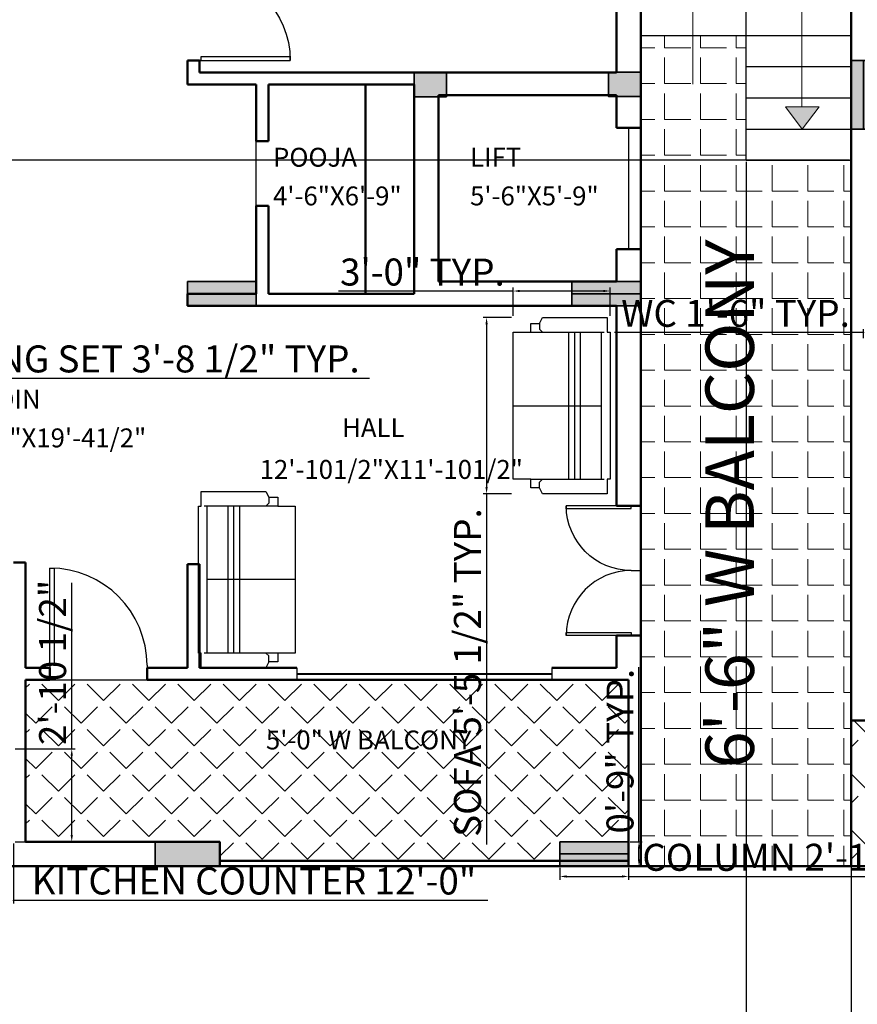
# Model space of a CAD drawing. Units: inches. Extents: x 2214 to 3937, y 762 to 2085.
# Tile 5 of 9: x 2933 to 3243, y 1424 to 1789. Entities that reach past the tile are written whole.
import ezdxf

# ---------------------------------------------------------------- set-up
doc = ezdxf.new("R2010")
doc.units = ezdxf.units.IN
for name, color, linetype, lineweight in [('A-ANNO-SYMB', 6, 'Continuous', 18), ('A-AREA-IDEN', 7, 'Continuous', 25), ('A-COLS', 5, 'Continuous', 35), ('A-COLS-PATT', 5, 'Continuous', 18), ('A-FLOR-PATT', 116, 'Continuous', 13), ('A-FURN', 8, 'Continuous', 18), ('C-ANNO-DIMS', 2, 'Continuous', 18), ('door', 122, 'Continuous', 25), ('stairs', 6, 'Continuous', 25), ('wall', 20, 'Continuous', 50), ('window', 4, 'Continuous', 25)]:
    doc.layers.add(name, color=color, linetype=linetype, lineweight=lineweight)
doc.layers.add('NOITHAT', color=21, linetype='Continuous')
doc.styles.get("Standard").update_dxf_attribs({"font": 'arial.ttf'})
doc.dimstyles.new('ISO-25', dxfattribs={"dimtxt": 10, "dimasz": 2.5, "dimexe": 1.25, "dimexo": 0.625, "dimtad": 1, "dimdec": 1, "dimlunit": 4, "dimtxsty": 'Standard', "dimcen": 2.5, "dimadec": 0, "dimazin": 0, "dimtfac": 1, "dimtdec": 1, "dimtmove": 0, "dimatfit": 3, "dimfxl": 1, "dimarcsym": 0})

# ---------------------------------------------------------------- blocks, each defined once
blk = doc.blocks.new('*U2')
for p, q in [((0, 0), (0, -6)), ((40, 0), (40, -6))]:
    blk.add_line(p, q)
blk.add_lwpolyline([(0, 0), (0, 40), (1.75, 40), (1.75, 0)], close=True)
blk.add_arc((0, 0), 40, 0, 90)
blk = doc.blocks.new('A$C0F740E5B')
at = {"layer": 'NOITHAT'}
for p, q in [((480, 1160), (480, 1120)), ((460, 1100), (40, 1100)), ((60, 100), (60, 1100)), ((200, 1100), (200, 100)), ((240, 1100), (240, 100)), ((280, 1100), (280, 100)), ((480, 1120), (460, 1100)), ((540, 1100), (460, 1100)), ((660, 600), (60, 600)), ((460, 100), (40, 100)), ((480, 80), (460, 100)), ((540, 100), (460, 100)), ((480, 40), (480, 80))]:
    blk.add_line(p, q, dxfattribs=at)
blk.add_lwpolyline([(20, 0), (20, 100), (0, 100), (0, 1100), (20, 1100), (20, 1200), (460, 1200), (480, 1160), (540, 1160), (540, 1100), (660, 1100), (660, 100), (540, 100), (540, 40), (480, 40), (460, 0)], close=True, dxfattribs=at)
blk = doc.blocks.new('COL-25_5X9')
at = {"ltscale": 0.3}
h = blk.add_hatch(color=256, dxfattribs=at)
h.dxf.hatch_style = 1
h.paths.add_polyline_path([(25.5, 0), (25.5, 9), (0, 9), (0, 0)])
for p, q in [((25.5, 9), (25.5, 0)), ((0, 4.5), (25.5, 4.5)), ((0, 4.5), (0, 0)), ((0, 0), (4.5, 0))]:
    blk.add_line(p, q)
blk.add_lwpolyline([(0, 9), (25.5, 9), (25.5, 0), (0, 0)], close=True, dxfattribs=at)
blk = doc.blocks.new('COL-12X9')
at = {"ltscale": 0.3}
h = blk.add_hatch(color=256, dxfattribs=at)
h.dxf.hatch_style = 1
h.paths.add_polyline_path([(12, 0), (12, 9), (0, 9), (0, 0)])
blk.add_lwpolyline([(12, 0), (0, 0), (0, 9), (12, 9)], close=True, dxfattribs=at)
blk = doc.blocks.new('*D33')
at = {"layer": 'C-ANNO-DIMS', "color": 0, "lineweight": -2, "ltscale": 0.3, "transparency": 16777216}
for p, q in [((3133.06, 1474.59), (3133.06, 1470.14)), ((3158.56, 1474.59), (3158.56, 1470.14)), ((3135.56, 1471.39), (3156.06, 1471.39)), ((3158.56, 1471.39), (3310.87, 1471.39))]:
    blk.add_line(p, q, dxfattribs=at)
at = {"layer": 'C-ANNO-DIMS', "color": 0, "ltscale": 0.3, "transparency": 16777216}
for points in [[(3135.56, 1471.81), (3135.56, 1470.98), (3133.06, 1471.39)], [(3156.06, 1471.81), (3156.06, 1470.98), (3158.56, 1471.39)]]:
    blk.add_solid(points, dxfattribs=at)
at = {"layer": 'Defpoints', "color": 0, "ltscale": 0.3, "transparency": 16777216}
for p in [(3133.06, 1475.22), (3158.56, 1475.22), (3158.56, 1471.39)]:
    blk.add_point(p, dxfattribs=at)
at = {"layer": 'C-ANNO-DIMS', "color": 0, "ltscale": 0.3, "transparency": 16777216, "insert": (3235.96, 1477.19), "char_height": 10, "attachment_point": 5}
blk.add_mtext('COLUMN 2\'-1 1/2" TYP.', dxfattribs=at)
blk = doc.blocks.new('*D34')
at = {"layer": 'C-ANNO-DIMS', "color": 0, "lineweight": -2, "ltscale": 0.3, "transparency": 16777216}
for p, q in [((3162.38, 1484.22), (3162.38, 1548.92)), ((3159.18, 1484.22), (3163.63, 1484.22)), ((3162.38, 1477.72), (3162.38, 1481.72)), ((3159.18, 1475.22), (3163.63, 1475.22))]:
    blk.add_line(p, q, dxfattribs=at)
at = {"layer": 'C-ANNO-DIMS', "color": 0, "ltscale": 0.3, "transparency": 16777216}
for points in [[(3161.97, 1481.72), (3162.8, 1481.72), (3162.38, 1484.22)], [(3161.97, 1477.72), (3162.8, 1477.72), (3162.38, 1475.22)]]:
    blk.add_solid(points, dxfattribs=at)
at = {"layer": 'Defpoints', "color": 0, "ltscale": 0.3, "transparency": 16777216}
for p in [(3158.56, 1484.22), (3162.38, 1484.22), (3158.56, 1475.22)]:
    blk.add_point(p, dxfattribs=at)
at = {"layer": 'C-ANNO-DIMS', "color": 0, "ltscale": 0.3, "transparency": 16777216, "insert": (3156.65, 1517.82), "char_height": 10, "attachment_point": 5, "rotation": 90}
blk.add_mtext('0\'-9" TYP.', dxfattribs=at)
blk = doc.blocks.new('*D49')
at = {"layer": 'C-ANNO-DIMS', "color": 0, "lineweight": -2, "ltscale": 0.3, "transparency": 16777216}
for p, q in [((3245.56, 1672.91), (3153.29, 1672.91)), ((3245.56, 1670.86), (3245.56, 1674.16)), ((3260.89, 1672.91), (3248.06, 1672.91)), ((3263.39, 1670.86), (3263.39, 1674.16))]:
    blk.add_line(p, q, dxfattribs=at)
at = {"layer": 'C-ANNO-DIMS', "color": 0, "ltscale": 0.3, "transparency": 16777216}
for points in [[(3248.06, 1673.33), (3248.06, 1672.5), (3245.56, 1672.91)], [(3260.89, 1673.33), (3260.89, 1672.5), (3263.39, 1672.91)]]:
    blk.add_solid(points, dxfattribs=at)
at = {"layer": 'Defpoints', "color": 0, "ltscale": 0.3, "transparency": 16777216}
for p in [(3245.56, 1672.91), (3245.56, 1670.24), (3263.39, 1670.24)]:
    blk.add_point(p, dxfattribs=at)
at = {"layer": 'C-ANNO-DIMS', "color": 0, "ltscale": 0.3, "transparency": 16777216, "insert": (3198.17, 1678.71), "char_height": 10, "attachment_point": 5}
blk.add_mtext('WC 1\'-6" TYP.', dxfattribs=at)
blk = doc.blocks.new('*D50')
at = {"layer": 'C-ANNO-DIMS', "color": 0, "lineweight": -2, "ltscale": 0.3, "transparency": 16777216}
for p, q in [((3266.06, 1670.24), (3266.06, 1757.3)), ((3264.01, 1670.24), (3267.31, 1670.24)), ((3266.06, 1660), (3266.06, 1667.74)), ((3264.01, 1657.5), (3267.31, 1657.5))]:
    blk.add_line(p, q, dxfattribs=at)
at = {"layer": 'C-ANNO-DIMS', "color": 0, "ltscale": 0.3, "transparency": 16777216}
for points in [[(3265.65, 1667.74), (3266.48, 1667.74), (3266.06, 1670.24)], [(3265.65, 1660), (3266.48, 1660), (3266.06, 1657.5)]]:
    blk.add_solid(points, dxfattribs=at)
at = {"layer": 'Defpoints', "color": 0, "ltscale": 0.3, "transparency": 16777216}
for p in [(3263.39, 1670.24), (3266.06, 1670.24), (3263.39, 1657.5)]:
    blk.add_point(p, dxfattribs=at)
at = {"layer": 'C-ANNO-DIMS', "color": 0, "ltscale": 0.3, "transparency": 16777216, "insert": (3260.27, 1715.02), "char_height": 10, "attachment_point": 5, "rotation": 90}
blk.add_mtext('1\'-0 1/2" TYP.', dxfattribs=at)
blk = doc.blocks.new('*D51')
at = {"layer": 'C-ANNO-DIMS', "color": 0, "lineweight": -2, "ltscale": 0.3, "transparency": 16777216}
for p, q in [((2846.77, 1662.06), (2846.77, 1654.77)), ((2891.18, 1662.06), (2891.18, 1654.77)), ((2849.27, 1656.02), (2888.68, 1656.02)), ((2891.18, 1656.02), (3062.52, 1656.02))]:
    blk.add_line(p, q, dxfattribs=at)
at = {"layer": 'C-ANNO-DIMS', "color": 0, "ltscale": 0.3, "transparency": 16777216}
for points in [[(2849.27, 1656.44), (2849.27, 1655.61), (2846.77, 1656.02)], [(2888.68, 1656.44), (2888.68, 1655.61), (2891.18, 1656.02)]]:
    blk.add_solid(points, dxfattribs=at)
at = {"layer": 'Defpoints', "color": 0, "ltscale": 0.3, "transparency": 16777216}
for p in [(2846.77, 1662.69), (2891.18, 1662.69), (2891.18, 1656.02)]:
    blk.add_point(p, dxfattribs=at)
at = {"layer": 'C-ANNO-DIMS', "color": 0, "ltscale": 0.3, "transparency": 16777216, "insert": (2978.1, 1661.82), "char_height": 10, "attachment_point": 5}
blk.add_mtext('DINING SET 3\'-8 1/2" TYP.', dxfattribs=at)
blk = doc.blocks.new('*D55')
at = {"layer": 'C-ANNO-DIMS', "color": 0, "lineweight": -2, "ltscale": 0.3, "transparency": 16777216}
for p, q in [((2786.56, 1483.59), (2786.56, 1461.37)), ((2930.56, 1483.59), (2930.56, 1461.37)), ((2789.06, 1462.62), (2928.06, 1462.62)), ((2930.56, 1462.62), (3106.37, 1462.62))]:
    blk.add_line(p, q, dxfattribs=at)
at = {"layer": 'C-ANNO-DIMS', "color": 0, "ltscale": 0.3, "transparency": 16777216}
for points in [[(2789.06, 1463.04), (2789.06, 1462.2), (2786.56, 1462.62)], [(2928.06, 1463.04), (2928.06, 1462.2), (2930.56, 1462.62)]]:
    blk.add_solid(points, dxfattribs=at)
at = {"layer": 'Defpoints', "color": 0, "ltscale": 0.3, "transparency": 16777216}
for p in [(2786.56, 1484.22), (2930.56, 1484.22), (2930.56, 1462.62)]:
    blk.add_point(p, dxfattribs=at)
at = {"layer": 'C-ANNO-DIMS', "color": 0, "ltscale": 0.3, "transparency": 16777216, "insert": (3019.71, 1468.42), "char_height": 10, "attachment_point": 5}
blk.add_mtext('KITCHEN COUNTER 12\'-0"', dxfattribs=at)
blk = doc.blocks.new('*D56')
at = {"layer": 'C-ANNO-DIMS', "color": 0, "lineweight": -2, "ltscale": 0.3, "transparency": 16777216}
for p, q in [((2952.16, 1518.65), (2952.16, 1580.23)), ((2931.18, 1518.65), (2953.41, 1518.65)), ((2952.16, 1486.72), (2952.16, 1516.15)), ((2931.18, 1484.22), (2953.41, 1484.22))]:
    blk.add_line(p, q, dxfattribs=at)
at = {"layer": 'C-ANNO-DIMS', "color": 0, "ltscale": 0.3, "transparency": 16777216}
for points in [[(2951.74, 1516.15), (2952.57, 1516.15), (2952.16, 1518.65)], [(2951.74, 1486.72), (2952.57, 1486.72), (2952.16, 1484.22)]]:
    blk.add_solid(points, dxfattribs=at)
at = {"layer": 'Defpoints', "color": 0, "ltscale": 0.3, "transparency": 16777216}
for p in [(2930.56, 1518.65), (2952.16, 1518.65), (2930.56, 1484.22)]:
    blk.add_point(p, dxfattribs=at)
at = {"layer": 'C-ANNO-DIMS', "color": 0, "ltscale": 0.3, "transparency": 16777216, "insert": (2946.36, 1550.69), "char_height": 10, "attachment_point": 5, "rotation": 90}
blk.add_mtext('2\'-10 1/2"', dxfattribs=at)
blk = doc.blocks.new('*D57')
at = {"layer": 'C-ANNO-DIMS', "color": 0, "lineweight": -2, "ltscale": 0.3, "transparency": 16777216}
for p, q in [((3115.09, 1678.47), (3104.66, 1678.47)), ((3105.91, 1675.97), (3105.91, 1615.63)), ((3115.09, 1613.13), (3104.66, 1613.13)), ((3105.91, 1613.13), (3105.91, 1483.25))]:
    blk.add_line(p, q, dxfattribs=at)
at = {"layer": 'C-ANNO-DIMS', "color": 0, "ltscale": 0.3, "transparency": 16777216}
for points in [[(3105.5, 1675.97), (3106.33, 1675.97), (3105.91, 1678.47)], [(3105.5, 1615.63), (3106.33, 1615.63), (3105.91, 1613.13)]]:
    blk.add_solid(points, dxfattribs=at)
at = {"layer": 'Defpoints', "color": 0, "ltscale": 0.3, "transparency": 16777216}
for p in [(3115.71, 1678.47), (3105.91, 1613.13), (3115.71, 1613.13)]:
    blk.add_point(p, dxfattribs=at)
at = {"layer": 'C-ANNO-DIMS', "color": 0, "ltscale": 0.3, "transparency": 16777216, "insert": (3100.11, 1546.94), "char_height": 10, "attachment_point": 5, "rotation": 90}
blk.add_mtext('SOFA 5\'-5 1/2" TYP.', dxfattribs=at)
blk = doc.blocks.new('*D58')
at = {"layer": 'C-ANNO-DIMS', "color": 0, "lineweight": -2, "ltscale": 0.3, "transparency": 16777216}
for p, q in [((3115.71, 1679.1), (3115.71, 1689.52)), ((3151.65, 1679.1), (3151.65, 1689.52)), ((3115.71, 1688.27), (3051.02, 1688.27)), ((3149.15, 1688.27), (3118.21, 1688.27))]:
    blk.add_line(p, q, dxfattribs=at)
at = {"layer": 'C-ANNO-DIMS', "color": 0, "ltscale": 0.3, "transparency": 16777216}
for points in [[(3118.21, 1688.69), (3118.21, 1687.86), (3115.71, 1688.27)], [(3149.15, 1688.69), (3149.15, 1687.86), (3151.65, 1688.27)]]:
    blk.add_solid(points, dxfattribs=at)
at = {"layer": 'Defpoints', "color": 0, "ltscale": 0.3, "transparency": 16777216}
for p in [(3115.71, 1688.27), (3115.71, 1678.47), (3151.65, 1678.47)]:
    blk.add_point(p, dxfattribs=at)
at = {"layer": 'C-ANNO-DIMS', "color": 0, "ltscale": 0.3, "transparency": 16777216, "insert": (3082.12, 1694.01), "char_height": 10, "attachment_point": 5}
blk.add_mtext('3\'-0" TYP.', dxfattribs=at)
blk = doc.blocks.new('*D63')
at = {"layer": 'C-ANNO-DIMS', "color": 0, "lineweight": -2, "ltscale": 0.3, "transparency": 16777216}
for p, q in [((3240.43, 1875.72), (2225.23, 1875.72)), ((2226.48, 1873.22), (2226.48, 1739.22)), ((3240.43, 1736.72), (2225.23, 1736.72))]:
    blk.add_line(p, q, dxfattribs=at)
at = {"layer": 'C-ANNO-DIMS', "color": 0, "ltscale": 0.3, "transparency": 16777216}
for points in [[(2226.07, 1873.22), (2226.9, 1873.22), (2226.48, 1875.72)], [(2226.07, 1739.22), (2226.9, 1739.22), (2226.48, 1736.72)]]:
    blk.add_solid(points, dxfattribs=at)
at = {"layer": 'Defpoints', "color": 0, "ltscale": 0.3, "transparency": 16777216}
for p in [(3241.06, 1875.72), (2226.48, 1736.72), (3241.06, 1736.72)]:
    blk.add_point(p, dxfattribs=at)
at = {"layer": 'C-ANNO-DIMS', "color": 0, "ltscale": 0.3, "transparency": 16777216, "insert": (2220.84, 1806.22), "char_height": 10, "attachment_point": 5, "rotation": 90}
blk.add_mtext('11\'-7"', dxfattribs=at)
blk = doc.blocks.new('*D64')
at = {"layer": 'C-ANNO-DIMS', "color": 0, "lineweight": -2, "ltscale": 0.3, "transparency": 16777216}
for p, q in [((3202.06, 1736.09), (3202.06, 792.32)), ((3241.06, 1736.09), (3241.06, 792.32)), ((3204.56, 793.57), (3238.56, 793.57))]:
    blk.add_line(p, q, dxfattribs=at)
at = {"layer": 'C-ANNO-DIMS', "color": 0, "ltscale": 0.3, "transparency": 16777216}
for points in [[(3204.56, 793.99), (3204.56, 793.15), (3202.06, 793.57)], [(3238.56, 793.99), (3238.56, 793.15), (3241.06, 793.57)]]:
    blk.add_solid(points, dxfattribs=at)
at = {"layer": 'Defpoints', "color": 0, "ltscale": 0.3, "transparency": 16777216}
for p in [(3202.06, 1736.72), (3241.06, 1736.72), (3241.06, 793.57)]:
    blk.add_point(p, dxfattribs=at)
at = {"layer": 'C-ANNO-DIMS', "color": 0, "ltscale": 0.3, "transparency": 16777216, "insert": (3221.56, 799.3), "char_height": 10, "attachment_point": 5}
blk.add_mtext('3\'-3"', dxfattribs=at)

msp = doc.modelspace()

# ---------------------------------------------------------------- hatches: boundary and pattern name
at = {"layer": 'A-ANNO-SYMB', "ltscale": 0.3}
h = msp.add_hatch(color=256, dxfattribs=at)
h.dxf.hatch_style = 1
h.paths.add_polyline_path([(3229.14, 1756.48), (3222.71, 1756.48), (3216.66, 1756.48), (3222.9, 1748.22)])
at = {"layer": 'A-COLS-PATT', "ltscale": 0.3}
h = msp.add_hatch(color=256, dxfattribs=at)
h.dxf.hatch_style = 1
h.paths.add_polyline_path([(3091.06, 1769.22), (3079.06, 1769.22), (3079.06, 1760.22), (3091.06, 1760.22)])
h = msp.add_hatch(color=256, dxfattribs=at)
h.dxf.hatch_style = 1
h.paths.add_polyline_path([(3020.56, 1682.78), (3020.56, 1691.78), (2995.06, 1691.78), (2995.06, 1682.78)])
h = msp.add_hatch(color=256, dxfattribs=at)
h.dxf.hatch_style = 1
h.paths.add_polyline_path([(3007.06, 1475.22), (3007.06, 1484.22), (2983.06, 1484.22), (2983.06, 1475.22)])
at = {"layer": 'A-FLOR-PATT', "ltscale": 0.3}
h = msp.add_hatch(dxfattribs=at)
h.set_pattern_fill('ANGLE', color=256, scale=1.9)
h.set_pattern_definition([(0, (0, 0), (0, 13.2715), [9.652, -3.6195]), (90, (0, 0), (-13.2715, 8e-16), [9.652, -3.6195])])
h.paths.add_polyline_path([(3241.06, 1736.72), (3202.06, 1736.72), (3202.06, 1782.99), (3163.06, 1782.99), (3163.06, 1475.22), (3241.06, 1475.22)])
h = msp.add_hatch(dxfattribs=at)
h.set_pattern_fill('ANGLE', color=256, scale=1.7, angle=45)
h.set_pattern_definition([(45, (0, 0), (-8.39654, 8.39654), [8.636, -3.2385]), (135, (0, 0), (-8.39654, -8.39654), [8.636, -3.2385])])
h.paths.add_polyline_path([(3158.56, 1544.22), (2980.06, 1544.22), (2944.06, 1544.22), (2935.06, 1544.22), (2935.06, 1484.22), (3007.06, 1484.22), (3007.06, 1477.24), (3133.06, 1477.24), (3133.06, 1484.22), (3158.56, 1484.22)])
h = msp.add_hatch(dxfattribs=at)
h.set_pattern_fill('ANGLE', color=256, scale=2.1, angle=45)
h.set_pattern_definition([(45, (0, 0), (-10.372196, 10.372196), [10.668, -4.0005]), (135, (0, 0), (-10.372196, -10.372196), [10.668, -4.0005])])
h.paths.add_polyline_path([(3571.06, 1529.18), (3562.06, 1529.18), (3241.06, 1529.22), (3241.06, 1475.22), (3571.06, 1475.22)])

# ---------------------------------------------------------------- linework, layer by layer
at = {"layer": 'A-ANNO-SYMB', "ltscale": 0.3}
for p, q in [((3182.33, 1764.86), (3182.33, 1889.49)), ((3222.71, 1889.49), (3222.71, 1756.48)), ((3223.09, 1756.48), (3216.66, 1756.48)), ((3216.66, 1756.48), (3222.9, 1748.22)), ((3222.71, 1756.48), (3229.14, 1756.48)), ((3229.14, 1756.48), (3222.9, 1748.22))]:
    msp.add_line(p, q, dxfattribs=at)
at = {"layer": 'A-COLS'}
msp.add_line((3020.56, 1691.78), (3020.56, 1682.78), dxfattribs=at)
at = {"layer": 'A-COLS', "ltscale": 0.3}
for points in [[(3091.06, 1760.22), (3079.06, 1760.22), (3079.06, 1769.22), (3091.06, 1769.22)], [(2995.06, 1691.78), (3020.56, 1691.78), (3020.56, 1682.78), (2995.06, 1682.78)], [(2983.06, 1484.22), (3007.06, 1484.22), (3007.06, 1475.22), (2983.06, 1475.22)]]:
    msp.add_lwpolyline(points, close=True, dxfattribs=at)
at = {"layer": 'door'}
for p, q in [((3158.56, 1748.78), (3158.56, 1703.78)), ((3020.56, 1719.84), (3020.56, 1743.84)), ((2944.06, 1544.22), (2980.06, 1544.22))]:
    msp.add_line(p, q, dxfattribs=at)
at = {"layer": 'stairs', "ltscale": 0.3}
for p, q in [((3202.06, 1736.72), (3202.06, 1875.72)), ((3163.06, 1782.99), (3241.06, 1782.99)), ((3202.06, 1771.4), (3241.06, 1771.4)), ((3202.06, 1759.81), (3241.06, 1759.81)), ((3202.06, 1748.22), (3241.06, 1748.22)), ((3202.06, 1736.72), (3241.06, 1736.72))]:
    msp.add_line(p, q, dxfattribs=at)
at = {"layer": 'wall'}
for p, q in [((3163.06, 1475.22), (3163.06, 1911.72)), ((3241.06, 1475.22), (3241.06, 1911.72)), ((3154.06, 1769.22), (3154.06, 1902.72)), ((2995.06, 1764.72), (2995.06, 1773.63)), ((2995.06, 1773.63), (2999.56, 1773.63)), ((2999.56, 1769.22), (2999.56, 1773.63)), ((2999.56, 1769.22), (3154.06, 1769.22)), ((2995.06, 1764.72), (3020.56, 1764.72)), ((3020.56, 1743.84), (3020.56, 1764.72)), ((3025.06, 1764.72), (3079.06, 1764.72)), ((3025.06, 1743.84), (3025.06, 1764.72)), ((3061.06, 1687.28), (3061.06, 1764.72)), ((3079.06, 1687.28), (3079.06, 1764.72)), ((3088.06, 1760.78), (3154.06, 1760.78)), ((3088.06, 1691.78), (3088.06, 1760.78)), ((3154.06, 1748.78), (3154.06, 1760.78)), ((3154.06, 1748.78), (3163.06, 1748.78)), ((3020.56, 1743.84), (3025.06, 1743.84)), ((3020.56, 1687.28), (3020.56, 1719.84)), ((3020.56, 1719.84), (3025.06, 1719.84)), ((3025.06, 1687.28), (3025.06, 1719.84)), ((3154.06, 1691.78), (3154.06, 1703.78)), ((3154.06, 1703.78), (3163.06, 1703.78)), ((3088.06, 1691.78), (3154.06, 1691.78)), ((2995.06, 1687.28), (3020.56, 1687.28)), ((2995.06, 1687.28), (2995.06, 1682.78)), ((3025.06, 1687.28), (3079.06, 1687.28)), ((2995.06, 1682.78), (2999.56, 1682.78)), ((2999.56, 1682.78), (3154.06, 1682.78)), ((3154.06, 1608.72), (3154.06, 1682.78)), ((3154.06, 1608.72), (3163.06, 1608.72)), ((2935.06, 1587.72), (2930.56, 1587.72)), ((2930.56, 1587.72), (2935.06, 1587.72)), ((2935.06, 1548.72), (2935.06, 1587.72)), ((2935.06, 1548.72), (2935.06, 1587.72)), ((2995.06, 1548.72), (2995.06, 1587.03)), ((2995.06, 1587.03), (2999.56, 1587.03)), ((2999.56, 1548.72), (2999.56, 1587.03)), ((3154.06, 1548.72), (3154.06, 1560.72)), ((3154.06, 1560.72), (3163.06, 1560.72)), ((2944.06, 1548.72), (2935.06, 1548.72)), ((2944.06, 1548.72), (2944.06, 1544.22)), ((2995.06, 1548.72), (2980.06, 1548.72)), ((2980.06, 1548.72), (2980.06, 1544.22)), ((3035.56, 1548.72), (2999.56, 1548.72)), ((3154.06, 1548.72), (3130.06, 1548.72)), ((2935.06, 1539.72), (2935.06, 1544.22)), ((2935.06, 1484.22), (2935.06, 1544.22)), ((2944.06, 1544.22), (2935.06, 1544.22)), ((3158.56, 1544.22), (2980.06, 1544.22)), ((3158.56, 1475.22), (3158.56, 1544.22)), ((2935.06, 1484.22), (2935.06, 1535.22)), ((3571.06, 1529.22), (3241.06, 1529.22)), ((3007.06, 1484.22), (2935.06, 1484.22)), ((3007.06, 1484.22), (3007.06, 1475.22)), ((3571.06, 1475.22), (2674.06, 1475.22)), ((3007.06, 1477.24), (3158.56, 1477.24))]:
    msp.add_line(p, q, dxfattribs=at)
at = {"layer": 'window'}
for p, q in [((3035.56, 1548.72), (3035.56, 1544.22)), ((3130.06, 1548.72), (3130.06, 1544.22)), ((3130.06, 1546.47), (3035.56, 1546.47)), ((3130.06, 1546.22), (3035.56, 1546.22))]:
    msp.add_line(p, q, dxfattribs=at)

# ---------------------------------------------------------------- block references
at = {"layer": 'A-COLS', "rotation": 270.0000000000005}
msp.add_blockref('COL-25_5X9', (3241.06, 1773.68), dxfattribs=at)
at = {"layer": 'A-COLS'}
for name, p in [('COL-12X9', (3151.06, 1760.36)), ('COL-25_5X9', (3137.56, 1682.78)), ('COL-25_5X9', (3133.06, 1475.22))]:
    msp.add_blockref(name, p, dxfattribs=at)
at = {"layer": 'A-FURN', "xscale": 0.0544503761205534, "yscale": 0.0544503761205534, "zscale": 0.0544503761205534, "rotation": 180}
msp.add_blockref('A$C0F740E5B', (3151.65, 1678.47), dxfattribs=at)
at = {"layer": 'A-FURN', "xscale": 0.0544503761205534, "yscale": 0.0544503761205534, "zscale": 0.0544503761205534}
msp.add_blockref('A$C0F740E5B', (2999.08, 1548.72), dxfattribs=at)
at = {"layer": 'door'}
for p, xscale, yscale, zscale, rotation in [((3000.02, 1773.63), -0.8273413149108705, 0.8273413149108705, 0.8273413149108705, 270), ((3159.46, 1608.72), -0.6, 0.6, 0.6, 90), ((3159.46, 1560.72), 0.6, 0.6, 0.6, 90)]:
    msp.add_blockref('*U2', p, dxfattribs=dict(at, xscale=xscale, yscale=yscale, zscale=zscale, rotation=rotation))
at = {"layer": 'door', "xscale": 0.9, "yscale": 0.9, "zscale": 0.9}
msp.add_blockref('*U2', (2944.06, 1549.62), dxfattribs=at)

# ---------------------------------------------------------------- texts
at = {"layer": 'A-AREA-IDEN', "ltscale": 0.3}
for s, p in [('POOJA', (3026.76, 1734.33)), ('LIFT', (3099.79, 1734.33)), ('4\'-6"X6\'-9"', (3026.76, 1720)), ('5\'-6"X5\'-9"', (3099.79, 1720)), ('LIV/DIN', (2907.16, 1644.69)), ('13\'-0"X19\'-41/2"', (2907.16, 1630.36)), ('HALL', (3052.37, 1634.17)), ('12\'-101/2"X11\'-101/2"', (3021.82, 1618.68)), ('5\'-0" W BALCONY', (3024.13, 1518.46))]:
    msp.add_text(s, height=7, dxfattribs=at).set_placement(p)
msp.add_text('6\'-6" W BALCONY', height=18, rotation=90, dxfattribs=at).set_placement((3205.01, 1511.47))

# ---------------------------------------------------------------- dimensions: what is measured, and where the dimension line sits
at = {"layer": 'C-ANNO-DIMS', "ltscale": 0.3}
for base, p1, p2, picture, middle in [((2226.48, 1736.72), (3241.06, 1875.72), (3241.06, 1736.72), '*D63', (2220.84, 1806.22)), ((2952.16, 1518.65), (2930.56, 1484.22), (2930.56, 1518.65), '*D56', (2946.36, 1550.69))]:
    dim = msp.add_linear_dim(base=base, p1=p1, p2=p2, angle=90, dimstyle='ISO-25', override={"dimdec": 1, "dimlfac": 1, "dimrnd": 0, "dimzin": 1, "dimdsep": 46, "dimlunit": 4, "dimfrac": 2}, dxfattribs=at)
    dim.commit()
    dim.dimension.update_dxf_attribs({"geometry": picture, "text_midpoint": middle})
for base, p1, p2, angle, text, picture, middle in [((3266.06, 1670.24), (3263.39, 1657.5), (3263.39, 1670.24), 90, '<> TYP.', '*D50', (3260.27, 1715.02)), ((3115.71, 1688.27), (3151.65, 1678.47), (3115.71, 1678.47), 180, '<> TYP.', '*D58', (3082.12, 1694.01)), ((3245.56, 1672.91), (3263.39, 1670.24), (3245.56, 1670.24), 180, 'WC <> TYP.', '*D49', (3198.17, 1678.71)), ((3105.91, 1613.13), (3115.71, 1678.47), (3115.71, 1613.13), 270, 'SOFA <> TYP.', '*D57', (3100.11, 1546.94)), ((3162.38, 1484.22), (3158.56, 1475.22), (3158.56, 1484.22), 90, '<> TYP.', '*D34', (3156.65, 1517.82))]:
    dim = msp.add_linear_dim(base=base, p1=p1, p2=p2, angle=angle, text=text, dimstyle='ISO-25', override={"dimdec": 1, "dimlfac": 1, "dimrnd": 0, "dimzin": 1, "dimdsep": 46, "dimlunit": 4, "dimfrac": 2}, dxfattribs=at)
    dim.commit()
    dim.dimension.update_dxf_attribs({"geometry": picture, "text_midpoint": middle})
dim = msp.add_linear_dim(base=(3241.06, 793.57), p1=(3202.06, 1736.72), p2=(3241.06, 1736.72), dimstyle='ISO-25', override={"dimdec": 1, "dimlfac": 1, "dimrnd": 0, "dimzin": 1, "dimdsep": 46, "dimlunit": 4, "dimfrac": 2}, dxfattribs=at)
dim.commit()
dim.dimension.update_dxf_attribs({"geometry": '*D64', "text_midpoint": (3221.56, 799.3)})
for base, p1, p2, text, picture, middle in [((2891.18, 1656.02), (2846.77, 1662.69), (2891.18, 1662.69), 'DINING SET <> TYP.', '*D51', (2978.1, 1661.82)), ((3158.56, 1471.39), (3133.06, 1475.22), (3158.56, 1475.22), 'COLUMN <> TYP.', '*D33', (3235.96, 1477.19)), ((2930.56, 1462.62), (2786.56, 1484.22), (2930.56, 1484.22), 'KITCHEN COUNTER <>', '*D55', (3019.71, 1468.42))]:
    dim = msp.add_linear_dim(base=base, p1=p1, p2=p2, text=text, dimstyle='ISO-25', override={"dimdec": 1, "dimlfac": 1, "dimrnd": 0, "dimzin": 1, "dimdsep": 46, "dimlunit": 4, "dimfrac": 2}, dxfattribs=at)
    dim.commit()
    dim.dimension.update_dxf_attribs({"geometry": picture, "text_midpoint": middle})

doc.saveas('drawing.dxf')
